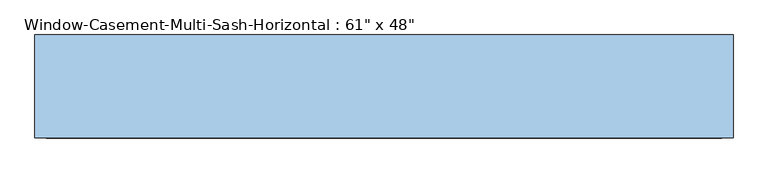
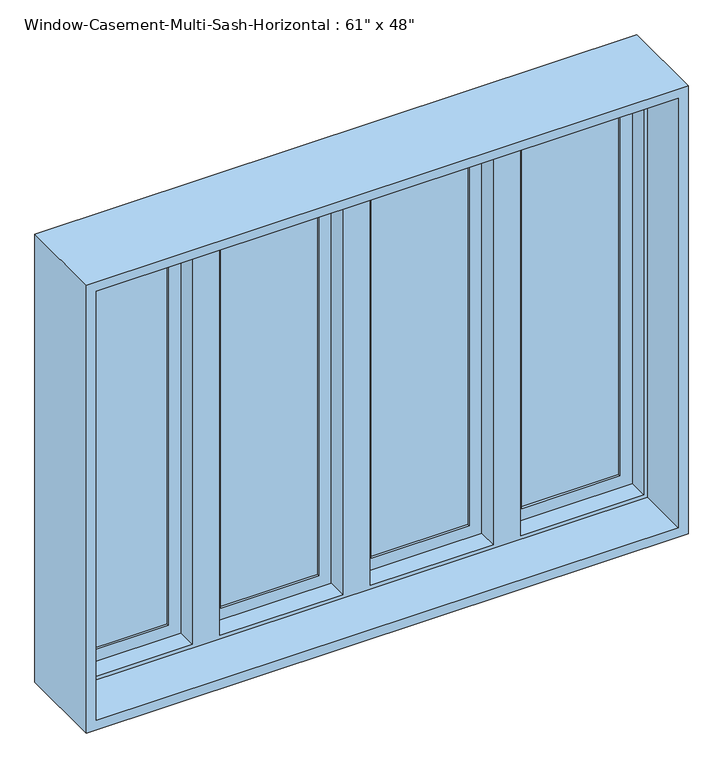
"""IFC4 building model written with IfcOpenShell, lengths in millimetres: window geometry."""

from ifc_helpers import new_model, si_unit, frame, origin, place, context, project, spatial, polyline, outline, extrude, faceted_brep, source, transform, mapped, element, save


def window_cf6260c5(model_context):
    return source(origin(), model_context, "Body", "SolidModel", [
        extrude(outline(polyline([(2108.2, 412.75), (939.8, 412.75), (939.8, 749.3), (2108.2, 749.3), (2108.2, 412.75)]), holes=[polyline([(2066.3296875, 707.4296875), (981.6703125, 707.4296875), (981.6703125, 454.6203125), (2066.3296875, 454.6203125), (2066.3296875, 707.4296875)])]), frame((0.0, 73.025, 0.0), z_axis=(0.0, 1.0, 0.0), x_axis=(0.0, 0.0, 1.0)), (0.0, 0.0, 1.0), 31.75),
        extrude(outline(polyline([(2108.2, -749.3), (939.8, -749.3), (939.8, -412.75), (2108.2, -412.75), (2108.2, -749.3)]), holes=[polyline([(2066.3296875, -454.6203125), (981.6703125, -454.6203125), (981.6703125, -707.4296875), (2066.3296875, -707.4296875), (2066.3296875, -454.6203125)])]), frame((0.0, 73.025, 0.0), z_axis=(0.0, 1.0, 0.0), x_axis=(0.0, 0.0, 1.0)), (0.0, 0.0, 1.0), 31.75),
        extrude(outline(polyline([(-454.6203125, 98.425), (-454.6203125, 92.075), (-707.4296875, 92.075), (-707.4296875, 98.425), (-454.6203125, 98.425)])), frame((0.0, 0.0, 981.6703125), z_axis=(0.0, 0.0, 1.0), x_axis=(1.0, 0.0, 0.0)), (0.0, 0.0, 1.0), 1084.659375),
        extrude(outline(polyline([(-454.6203125, 85.725), (-454.6203125, 79.375), (-707.4296875, 79.375), (-707.4296875, 85.725), (-454.6203125, 85.725)])), frame((0.0, 0.0, 981.6703125), z_axis=(0.0, 0.0, 1.0), x_axis=(1.0, 0.0, 0.0)), (0.0, 0.0, 1.0), 1084.659375),
        extrude(outline(polyline([(707.4296875, 98.425), (707.4296875, 92.075), (454.6203125, 92.075), (454.6203125, 98.425), (707.4296875, 98.425)])), frame((0.0, 0.0, 981.6703125), z_axis=(0.0, 0.0, 1.0), x_axis=(1.0, 0.0, 0.0)), (0.0, 0.0, 1.0), 1084.659375),
        extrude(outline(polyline([(707.4296875, 85.725), (707.4296875, 79.375), (454.6203125, 79.375), (454.6203125, 85.725), (707.4296875, 85.725)])), frame((0.0, 0.0, 981.6703125), z_axis=(0.0, 0.0, 1.0), x_axis=(1.0, 0.0, 0.0)), (0.0, 0.0, 1.0), 1084.659375),
        extrude(outline(polyline([(-67.2703125, 98.425), (-67.2703125, 92.075), (-320.0796875, 92.075), (-320.0796875, 98.425), (-67.2703125, 98.425)])), frame((0.0, 0.0, 981.6703125), z_axis=(0.0, 0.0, 1.0), x_axis=(1.0, 0.0, 0.0)), (0.0, 0.0, 1.0), 1084.659375),
        extrude(outline(polyline([(-67.2703125, 85.725), (-67.2703125, 79.375), (-320.0796875, 79.375), (-320.0796875, 85.725), (-67.2703125, 85.725)])), frame((0.0, 0.0, 981.6703125), z_axis=(0.0, 0.0, 1.0), x_axis=(1.0, 0.0, 0.0)), (0.0, 0.0, 1.0), 1084.659375),
        extrude(outline(polyline([(320.0796875, 98.425), (320.0796875, 92.075), (67.2703125, 92.075), (67.2703125, 98.425), (320.0796875, 98.425)])), frame((0.0, 0.0, 981.6703125), z_axis=(0.0, 0.0, 1.0), x_axis=(1.0, 0.0, 0.0)), (0.0, 0.0, 1.0), 1084.659375),
        extrude(outline(polyline([(320.0796875, 85.725), (320.0796875, 79.375), (67.2703125, 79.375), (67.2703125, 85.725), (320.0796875, 85.725)])), frame((0.0, 0.0, 981.6703125), z_axis=(0.0, 0.0, 1.0), x_axis=(1.0, 0.0, 0.0)), (0.0, 0.0, 1.0), 1084.659375),
        faceted_brep([(-412.75, 73.025, 2108.2), (-749.3, 73.025, 2108.2), (-749.3, 114.3, 2108.2), (749.3, 114.3, 2108.2), (749.3, 73.025, 2108.2), (412.75, 73.025, 2108.2), (412.75, 111.125, 2108.2), (361.95, 111.125, 2108.2), (361.95, 73.025, 2108.2), (25.4, 73.025, 2108.2), (25.4, 111.125, 2108.2), (-25.4, 111.125, 2108.2), (-25.4, 73.025, 2108.2), (-361.95, 73.025, 2108.2), (-361.95, 111.125, 2108.2), (-412.75, 111.125, 2108.2), (-739.1796875, 22.225, 2098.0796875), (-739.1796875, 73.025, 2098.0796875), (-422.8703125, 73.025, 2098.0796875), (-422.8703125, 22.225, 2098.0796875), (739.1796875, 73.025, 2098.0796875), (739.1796875, 22.225, 2098.0796875), (422.8703125, 22.225, 2098.0796875), (422.8703125, 73.025, 2098.0796875), (-351.8296875, 73.025, 2098.0796875), (-35.5203125, 73.025, 2098.0796875), (-35.5203125, 22.225, 2098.0796875), (-351.8296875, 22.225, 2098.0796875), (35.5203125, 73.025, 2098.0796875), (351.8296875, 73.025, 2098.0796875), (351.8296875, 22.225, 2098.0796875), (35.5203125, 22.225, 2098.0796875), (-749.3, -114.3, 2108.2), (-749.3, 22.225, 2108.2), (749.3, 22.225, 2108.2), (749.3, -114.3, 2108.2), (-774.7, 114.3, 2133.6), (-774.7, -114.3, 2133.6), (774.7, -114.3, 2133.6), (774.7, 114.3, 2133.6), (749.3, 114.3, 939.8), (749.3, 73.025, 939.8), (739.1796875, 73.025, 949.9203125), (739.1796875, 22.225, 949.9203125), (749.3, 22.225, 939.8), (749.3, -114.3, 939.8), (774.7, -114.3, 914.4), (774.7, 114.3, 914.4), (412.75, 73.025, 939.8), (-749.3, 114.3, 939.8), (-749.3, 73.025, 939.8), (-412.75, 73.025, 939.8), (-412.75, 111.125, 939.8), (-361.95, 111.125, 939.8), (-361.95, 73.025, 939.8), (-25.4, 73.025, 939.8), (-25.4, 111.125, 939.8), (25.4, 111.125, 939.8), (25.4, 73.025, 939.8), (361.95, 73.025, 939.8), (361.95, 111.125, 939.8), (412.75, 111.125, 939.8), (422.8703125, 73.025, 949.9203125), (422.8703125, 22.225, 949.9203125), (-739.1796875, 73.025, 949.9203125), (-739.1796875, 22.225, 949.9203125), (-422.8703125, 22.225, 949.9203125), (-422.8703125, 73.025, 949.9203125), (-35.5203125, 73.025, 949.9203125), (-351.8296875, 73.025, 949.9203125), (-351.8296875, 22.225, 949.9203125), (-35.5203125, 22.225, 949.9203125), (351.8296875, 73.025, 949.9203125), (35.5203125, 73.025, 949.9203125), (35.5203125, 22.225, 949.9203125), (351.8296875, 22.225, 949.9203125), (-749.3, 22.225, 939.8), (-749.3, -114.3, 939.8), (-774.7, -114.3, 914.4), (-774.7, 114.3, 914.4)], [[[0, 1, 2, 3, 4, 5, 6, 7, 8, 9, 10, 11, 12, 13, 14, 15]], [[16, 17, 18, 19]], [[20, 21, 22, 23]], [[24, 25, 26, 27]], [[28, 29, 30, 31]], [[32, 33, 34, 35]], [[36, 37, 38, 39]], [[4, 3, 40, 41]], [[21, 20, 42, 43]], [[35, 34, 44, 45]], [[39, 38, 46, 47]], [[48, 41, 40, 49, 50, 51, 52, 53, 54, 55, 56, 57, 58, 59, 60, 61]], [[43, 42, 62, 63]], [[64, 65, 66, 67]], [[68, 69, 70, 71]], [[72, 73, 74, 75]], [[45, 44, 76, 77]], [[47, 46, 78, 79]], [[2, 1, 50, 49]], [[4, 41, 48, 5], [20, 23, 62, 42]], [[50, 1, 0, 51], [64, 67, 18, 17]], [[12, 55, 54, 13], [69, 68, 25, 24]], [[8, 59, 58, 9], [73, 72, 29, 28]], [[17, 16, 65, 64]], [[44, 34, 33, 76], [16, 19, 66, 65], [27, 26, 71, 70], [31, 30, 75, 74], [21, 43, 63, 22]], [[33, 32, 77, 76]], [[38, 37, 78, 46], [32, 35, 45, 77]], [[37, 36, 79, 78]], [[36, 39, 47, 79], [3, 2, 49, 40]], [[18, 67, 66, 19]], [[69, 24, 27, 70]], [[53, 14, 13, 54]], [[14, 53, 52, 15]], [[15, 52, 51, 0]], [[25, 68, 71, 26]], [[73, 28, 31, 74]], [[57, 10, 9, 58]], [[10, 57, 56, 11]], [[11, 56, 55, 12]], [[6, 61, 60, 7]], [[7, 60, 59, 8]], [[29, 72, 75, 30]], [[62, 23, 22, 63]], [[61, 6, 5, 48]]]),
        extrude(outline(polyline([(2108.2, 25.4), (939.8, 25.4), (939.8, 361.95), (2108.2, 361.95), (2108.2, 25.4)]), holes=[polyline([(2066.3296875, 320.0796875), (981.6703125, 320.0796875), (981.6703125, 67.2703125), (2066.3296875, 67.2703125), (2066.3296875, 320.0796875)])]), frame((0.0, 73.025, 0.0), z_axis=(0.0, 1.0, 0.0), x_axis=(0.0, 0.0, 1.0)), (0.0, 0.0, 1.0), 31.75),
        extrude(outline(polyline([(2108.2, -361.95), (939.8, -361.95), (939.8, -25.4), (2108.2, -25.4), (2108.2, -361.95)]), holes=[polyline([(2066.3296875, -67.2703125), (981.6703125, -67.2703125), (981.6703125, -320.0796875), (2066.3296875, -320.0796875), (2066.3296875, -67.2703125)])]), frame((0.0, 73.025, 0.0), z_axis=(0.0, 1.0, 0.0), x_axis=(0.0, 0.0, 1.0)), (0.0, 0.0, 1.0), 31.75),
    ])


if __name__ == "__main__":
    model = new_model("IFC4")
    model_context = context("Model", 3, world=origin())
    ifc_project = project(units=[si_unit("LENGTHUNIT", "METRE", prefix="MILLI")], contexts=[model_context])
    site = spatial("IfcSite", under=ifc_project)
    building = spatial("IfcBuilding", under=site)
    placement = place(None, origin())
    window_shape = window_cf6260c5(model_context)
    element("IfcWindow", 1, ObjectType="Window-Casement-Multi-Sash-Horizontal : 61\" x 48\"", at=placement, inside=building, context=model_context, shape_type="MappedRepresentation", body=[
        mapped(window_shape, transform((0.0, 0.0, 0.0), x_axis=(1.0, 0.0, 0.0), y_axis=(0.0, 1.0, 0.0), z_axis=(0.0, 0.0, 1.0))),
    ])
    save(model, "model.ifc")

# Revit data of these elements
# Type "Window-Casement-Multi-Sash-Horizontal : 61\" x 48\""
#   Type Mark = "21"
#   Fire Rating = "0.5h"
#   Assembly Code = "B2020100"
#   Analytic Construction = "Double glazing - domestic"
#   Window Inset [instance default] = 0' - 0 5/8"
#   Wall Thickness [instance default] = 0' - 6"
#   Visual Light Transmittance = 0.81
#   Thermal Resistance (R) = 1.8146 (h·ft²·°F)/BTU
#   Solar Heat Gain Coefficient = 0.76
#   Rough Width = 5' - 1 1/2"
#   Rough Height = 4' - 0 1/2"
#   Open Window Width = 1' - 3 1/4"
#   Heat Transfer Coefficient (U) = 0.5511 BTU/(h·ft²·°F)
#   Height = 4' - 0"
#   Frame Gap 3 [instance default] = 0' - 1 83/128"
#   Frame Gap 2 [instance default] = 0' - 0 5/8"
#   Frame Gap 1 = 0' - 1 51/128"
#   Default Sill Height = 3' - 0"
#   Width = 5' - 1"
#   Frame Material = Metal - Aluminum
#   Glass Panel Material = Glass
#   Wall Closure = (empty or 0)
# Element 1 (IfcWindow, "Window-Casement-Multi-Sash-Horizontal : 61\" x 48\"")
#   Wall Thickness = 0' - 9"
#   Materials on its faces: "Metal - Aluminum", "Glass"
# Materials
#   "Metal - Aluminum": class "Metal", colour RGB 247 247 247, transparency 0
#   "Glass": class "Glass", colour RGB 0 128 192, transparency 0.75, Description = "Soda Lime Glass", Cost = 0
